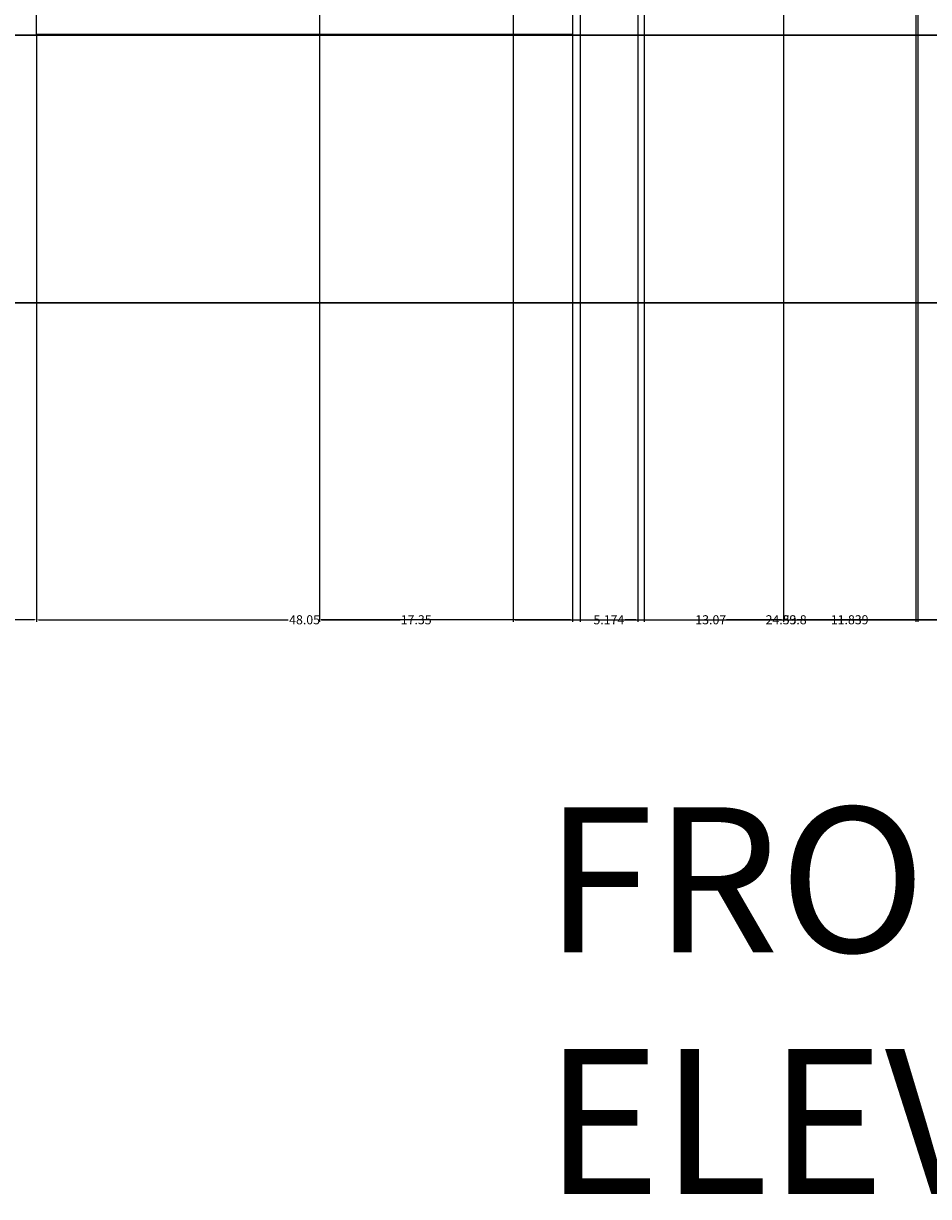
# Model space of a CAD drawing. Units: inches. Extents: x 69 to 650, y -16 to 573.
# Tile 4 of 26: x 264 to 345, y -16 to 89. Entities that reach past the tile are written whole.
import ezdxf

# ---------------------------------------------------------------- set-up
doc = ezdxf.new("R2010")
doc.units = ezdxf.units.IN
doc.header["$MEASUREMENT"] = 0
for name, color, linetype, lineweight in [('A-ANNO-DIMS', 2, 'Continuous', 18), ('A-ANNO-TEXT', 7, 'Continuous', 25), ('A-DOOR', 3, 'Continuous', 25), ('A-WALL-BASE', 7, 'Continuous', 30)]:
    doc.layers.add(name, color=color, linetype=linetype, lineweight=lineweight)
doc.styles.get("Standard").update_dxf_attribs({"font": 'arial.ttf'})
doc.dimstyles.get("Standard").update_dxf_attribs({"dimtxt": 0.8125, "dimasz": 0.18, "dimexe": 0.18, "dimexo": 0.0625, "dimgap": 0.09, "dimtad": 0, "dimtih": 1, "dimtoh": 1, "dimdec": 4, "dimzin": 0, "dimdsep": 46, "dimlunit": 4, "dimtxsty": 'Standard', "dimcen": 0.09, "dimadec": 0, "dimazin": 0, "dimtfac": 1, "dimtdec": 4, "dimtofl": 0, "dimtmove": 0, "dimatfit": 3, "dimfxl": 1, "dimtolj": 1, "dimtzin": 0, "dimarcsym": 0})

# ---------------------------------------------------------------- blocks, each defined once
blk = doc.blocks.new('*D19')
at = {"layer": 'A-ANNO-DIMS', "color": 0, "lineweight": -2, "transparency": 16777216}
for p, q in [((99.56, 471.72), (99.56, 572.74)), ((99.74, 572.56), (358.57, 572.56)), ((619.38, 572.56), (360.54, 572.56)), ((619.56, 87.99), (619.56, 572.74))]:
    blk.add_line(p, q, dxfattribs=at)
at = {"layer": 'A-ANNO-DIMS', "color": 0, "transparency": 16777216}
for points in [[(99.74, 572.59), (99.74, 572.53), (99.56, 572.56)], [(619.38, 572.59), (619.38, 572.53), (619.56, 572.56)]]:
    blk.add_solid(points, dxfattribs=at)
at = {"layer": 'Defpoints', "color": 0, "transparency": 16777216}
for p in [(619.56, 572.56), (99.56, 471.66), (619.56, 87.93)]:
    blk.add_point(p, dxfattribs=at)
at = {"layer": 'A-ANNO-DIMS', "color": 0, "transparency": 16777216, "insert": (359.56, 572.56), "char_height": 0.812, "attachment_point": 5}
blk.add_mtext('\\A1;520', dxfattribs=at)
blk = doc.blocks.new('*D28')
at = {"layer": 'A-ANNO-DIMS', "color": 0, "lineweight": -2, "transparency": 16777216}
for p, q in [((225, 87.87), (225, 35.35)), ((265.1, 87.92), (265.1, 35.35)), ((225.18, 35.53), (243.96, 35.53)), ((264.92, 35.53), (246.13, 35.53))]:
    blk.add_line(p, q, dxfattribs=at)
at = {"layer": 'A-ANNO-DIMS', "color": 0, "transparency": 16777216}
for points in [[(225.18, 35.56), (225.18, 35.5), (225, 35.53)], [(264.92, 35.56), (264.92, 35.5), (265.1, 35.53)]]:
    blk.add_solid(points, dxfattribs=at)
at = {"layer": 'Defpoints', "color": 0, "transparency": 16777216}
for p in [(225, 87.93), (265.1, 87.99), (265.1, 35.53)]:
    blk.add_point(p, dxfattribs=at)
at = {"layer": 'A-ANNO-DIMS', "color": 0, "transparency": 16777216, "insert": (245.05, 35.53), "char_height": 0.812, "attachment_point": 5}
blk.add_mtext('\\A1;40.1', dxfattribs=at)
blk = doc.blocks.new('*D29')
at = {"layer": 'A-ANNO-DIMS', "color": 0, "lineweight": -2, "transparency": 16777216}
for p, q in [((265.1, 87.92), (265.1, 35.35)), ((313.14, 87.92), (313.14, 35.35)), ((265.28, 35.53), (287.64, 35.53)), ((312.96, 35.53), (290.6, 35.53))]:
    blk.add_line(p, q, dxfattribs=at)
at = {"layer": 'A-ANNO-DIMS', "color": 0, "transparency": 16777216}
for points in [[(265.28, 35.56), (265.28, 35.5), (265.1, 35.53)], [(312.96, 35.56), (312.96, 35.5), (313.14, 35.53)]]:
    blk.add_solid(points, dxfattribs=at)
at = {"layer": 'Defpoints', "color": 0, "transparency": 16777216}
for p in [(265.1, 87.99), (313.14, 87.99), (313.14, 35.53)]:
    blk.add_point(p, dxfattribs=at)
at = {"layer": 'A-ANNO-DIMS', "color": 0, "transparency": 16777216, "insert": (289.12, 35.53), "char_height": 0.812, "attachment_point": 5}
blk.add_mtext('\\A1;48.05', dxfattribs=at)
blk = doc.blocks.new('*D30')
at = {"layer": 'A-ANNO-DIMS', "color": 0, "lineweight": -2, "transparency": 16777216}
for p, q in [((352.94, 174.2), (352.94, 35.35)), ((313.14, 87.92), (313.14, 35.35)), ((313.32, 35.53), (331.9, 35.53)), ((352.76, 35.53), (334.19, 35.53))]:
    blk.add_line(p, q, dxfattribs=at)
at = {"layer": 'A-ANNO-DIMS', "color": 0, "transparency": 16777216}
for points in [[(313.32, 35.56), (313.32, 35.5), (313.14, 35.53)], [(352.76, 35.56), (352.76, 35.5), (352.94, 35.53)]]:
    blk.add_solid(points, dxfattribs=at)
at = {"layer": 'Defpoints', "color": 0, "transparency": 16777216}
for p in [(352.94, 174.27), (313.14, 87.99), (352.94, 35.53)]:
    blk.add_point(p, dxfattribs=at)
at = {"layer": 'A-ANNO-DIMS', "color": 0, "transparency": 16777216, "insert": (333.04, 35.53), "char_height": 0.812, "attachment_point": 5}
blk.add_mtext('\\A1;39.8', dxfattribs=at)
blk = doc.blocks.new('*D37')
at = {"layer": 'A-ANNO-DIMS', "color": 0, "lineweight": -2, "transparency": 16777216}
for p, q in [((307.8, 384.84), (307.8, 35.35)), ((290.45, 372.93), (290.45, 35.35)), ((290.63, 35.53), (297.7, 35.53)), ((307.62, 35.53), (300.55, 35.53))]:
    blk.add_line(p, q, dxfattribs=at)
at = {"layer": 'A-ANNO-DIMS', "color": 0, "transparency": 16777216}
for points in [[(290.63, 35.56), (290.63, 35.5), (290.45, 35.53)], [(307.62, 35.56), (307.62, 35.5), (307.8, 35.53)]]:
    blk.add_solid(points, dxfattribs=at)
at = {"layer": 'Defpoints', "color": 0, "transparency": 16777216}
for p in [(307.8, 384.9), (290.45, 372.99), (307.8, 35.53)]:
    blk.add_point(p, dxfattribs=at)
at = {"layer": 'A-ANNO-DIMS', "color": 0, "transparency": 16777216, "insert": (299.12, 35.53), "char_height": 0.812, "attachment_point": 5}
blk.add_mtext('\\A1;17.35', dxfattribs=at)
blk = doc.blocks.new('*D38')
at = {"layer": 'A-ANNO-DIMS', "color": 0, "lineweight": -2, "transparency": 16777216}
for p, q in [((307.8, 384.84), (307.8, 35.35)), ((390.43, 384.84), (390.43, 35.35)), ((307.98, 35.53), (347.65, 35.53)), ((390.25, 35.53), (350.57, 35.53))]:
    blk.add_line(p, q, dxfattribs=at)
at = {"layer": 'A-ANNO-DIMS', "color": 0, "transparency": 16777216}
for points in [[(307.98, 35.56), (307.98, 35.5), (307.8, 35.53)], [(390.25, 35.56), (390.25, 35.5), (390.43, 35.53)]]:
    blk.add_solid(points, dxfattribs=at)
at = {"layer": 'Defpoints', "color": 0, "transparency": 16777216}
for p in [(307.8, 384.9), (390.43, 384.9), (390.43, 35.53)]:
    blk.add_point(p, dxfattribs=at)
at = {"layer": 'A-ANNO-DIMS', "color": 0, "transparency": 16777216, "insert": (349.11, 35.53), "char_height": 0.812, "attachment_point": 5}
blk.add_mtext('\\A1;82.63', dxfattribs=at)
blk = doc.blocks.new('*D64')
at = {"layer": 'A-ANNO-DIMS', "color": 0, "lineweight": -2, "transparency": 16777216}
for p, q in [((319.55, 393.8), (319.55, 35.35)), ((344.08, 393.8), (344.08, 35.35)), ((319.73, 35.53), (330.35, 35.53)), ((343.9, 35.53), (333.28, 35.53))]:
    blk.add_line(p, q, dxfattribs=at)
at = {"layer": 'A-ANNO-DIMS', "color": 0, "transparency": 16777216}
for points in [[(319.73, 35.56), (319.73, 35.5), (319.55, 35.53)], [(343.9, 35.56), (343.9, 35.5), (344.08, 35.53)]]:
    blk.add_solid(points, dxfattribs=at)
at = {"layer": 'Defpoints', "color": 0, "transparency": 16777216}
for p in [(319.55, 393.86), (344.08, 393.86), (344.08, 35.53)]:
    blk.add_point(p, dxfattribs=at)
at = {"layer": 'A-ANNO-DIMS', "color": 0, "transparency": 16777216, "insert": (331.82, 35.53), "char_height": 0.812, "attachment_point": 5}
blk.add_mtext('\\A1;24.53', dxfattribs=at)
blk = doc.blocks.new('*D65')
at = {"layer": 'A-ANNO-DIMS', "color": 0, "lineweight": -2, "transparency": 16777216}
for p, q in [((344.08, 393.8), (344.08, 35.35)), ((368.88, 393.8), (368.88, 35.35)), ((344.26, 35.53), (355.33, 35.53)), ((368.7, 35.53), (357.63, 35.53))]:
    blk.add_line(p, q, dxfattribs=at)
at = {"layer": 'A-ANNO-DIMS', "color": 0, "transparency": 16777216}
for points in [[(344.26, 35.56), (344.26, 35.5), (344.08, 35.53)], [(368.7, 35.56), (368.7, 35.5), (368.88, 35.53)]]:
    blk.add_solid(points, dxfattribs=at)
at = {"layer": 'Defpoints', "color": 0, "transparency": 16777216}
for p in [(344.08, 393.86), (368.88, 393.86), (368.88, 35.53)]:
    blk.add_point(p, dxfattribs=at)
at = {"layer": 'A-ANNO-DIMS', "color": 0, "transparency": 16777216, "insert": (356.48, 35.53), "char_height": 0.812, "attachment_point": 5}
blk.add_mtext('\\A1;24.8', dxfattribs=at)
blk = doc.blocks.new('*D66')
at = {"layer": 'A-ANNO-DIMS', "color": 0, "lineweight": -2, "transparency": 16777216}
for p, q in [((313.81, 263.46), (313.81, 35.35)), ((318.98, 263.46), (318.98, 35.35)), ((313.99, 35.53), (314.93, 35.53)), ((318.8, 35.53), (317.85, 35.53))]:
    blk.add_line(p, q, dxfattribs=at)
at = {"layer": 'A-ANNO-DIMS', "color": 0, "transparency": 16777216}
for points in [[(313.99, 35.56), (313.99, 35.5), (313.81, 35.53)], [(318.8, 35.56), (318.8, 35.5), (318.98, 35.53)]]:
    blk.add_solid(points, dxfattribs=at)
at = {"layer": 'Defpoints', "color": 0, "transparency": 16777216}
for p in [(313.81, 263.53), (318.98, 263.53), (318.98, 35.53)]:
    blk.add_point(p, dxfattribs=at)
at = {"layer": 'A-ANNO-DIMS', "color": 0, "transparency": 16777216, "insert": (316.39, 35.53), "char_height": 0.812, "attachment_point": 5}
blk.add_mtext('\\A1;5.174', dxfattribs=at)
blk = doc.blocks.new('*D67')
at = {"layer": 'A-ANNO-DIMS', "color": 0, "lineweight": -2, "transparency": 16777216}
for p, q in [((318.98, 263.46), (318.98, 35.35)), ((332.05, 263.46), (332.05, 35.35)), ((319.16, 35.53), (324.09, 35.53)), ((331.87, 35.53), (326.94, 35.53))]:
    blk.add_line(p, q, dxfattribs=at)
at = {"layer": 'A-ANNO-DIMS', "color": 0, "transparency": 16777216}
for points in [[(319.16, 35.56), (319.16, 35.5), (318.98, 35.53)], [(331.87, 35.56), (331.87, 35.5), (332.05, 35.53)]]:
    blk.add_solid(points, dxfattribs=at)
at = {"layer": 'Defpoints', "color": 0, "transparency": 16777216}
for p in [(318.98, 263.53), (332.05, 263.53), (332.05, 35.53)]:
    blk.add_point(p, dxfattribs=at)
at = {"layer": 'A-ANNO-DIMS', "color": 0, "transparency": 16777216, "insert": (325.52, 35.53), "char_height": 0.812, "attachment_point": 5}
blk.add_mtext('\\A1;13.07', dxfattribs=at)
blk = doc.blocks.new('*D68')
at = {"layer": 'A-ANNO-DIMS', "color": 0, "lineweight": -2, "transparency": 16777216}
for p, q in [((332.05, 263.46), (332.05, 35.35)), ((343.89, 263.46), (343.89, 35.35)), ((332.23, 35.53), (336.23, 35.53)), ((343.71, 35.53), (339.71, 35.53))]:
    blk.add_line(p, q, dxfattribs=at)
at = {"layer": 'A-ANNO-DIMS', "color": 0, "transparency": 16777216}
for points in [[(332.23, 35.56), (332.23, 35.5), (332.05, 35.53)], [(343.71, 35.56), (343.71, 35.5), (343.89, 35.53)]]:
    blk.add_solid(points, dxfattribs=at)
at = {"layer": 'Defpoints', "color": 0, "transparency": 16777216}
for p in [(332.05, 263.53), (343.89, 263.53), (343.89, 35.53)]:
    blk.add_point(p, dxfattribs=at)
at = {"layer": 'A-ANNO-DIMS', "color": 0, "transparency": 16777216, "insert": (337.97, 35.53), "char_height": 0.812, "attachment_point": 5}
blk.add_mtext('\\A1;11.839', dxfattribs=at)
blk = doc.blocks.new('*D69')
at = {"layer": 'A-ANNO-DIMS', "color": 0, "lineweight": -2, "transparency": 16777216}
for p, q in [((343.89, 263.46), (343.89, 35.35)), ((357.51, 263.46), (357.51, 35.35)), ((344.07, 35.53), (349.28, 35.53)), ((357.33, 35.53), (352.12, 35.53))]:
    blk.add_line(p, q, dxfattribs=at)
at = {"layer": 'A-ANNO-DIMS', "color": 0, "transparency": 16777216}
for points in [[(344.07, 35.56), (344.07, 35.5), (343.89, 35.53)], [(357.33, 35.56), (357.33, 35.5), (357.51, 35.53)]]:
    blk.add_solid(points, dxfattribs=at)
at = {"layer": 'Defpoints', "color": 0, "transparency": 16777216}
for p in [(343.89, 263.53), (357.51, 263.53), (357.51, 35.53)]:
    blk.add_point(p, dxfattribs=at)
at = {"layer": 'A-ANNO-DIMS', "color": 0, "transparency": 16777216, "insert": (350.7, 35.53), "char_height": 0.812, "attachment_point": 5}
blk.add_mtext('\\A1;13.62', dxfattribs=at)

msp = doc.modelspace()

# ---------------------------------------------------------------- linework, layer by layer
at = {"layer": 'A-DOOR'}
msp.add_lwpolyline([(265.0952, 174.2666), (313.1416, 174.2666), (313.1416, 87.985), (265.0952, 87.985)], close=True, dxfattribs=at)
at = {"layer": 'A-WALL-BASE'}
for p, q in [((99.556, 87.93), (463.7847, 87.93)), ((99.556, 63.93), (463.7847, 63.93))]:
    msp.add_line(p, q, dxfattribs=at)

# ---------------------------------------------------------------- texts
at = {"layer": 'A-ANNO-TEXT', "insert": (310.6022, 18.729), "char_height": 13, "attachment_point": 1}
msp.add_mtext_dynamic_manual_height_columns('FRONT ELEVATION', width=154.108417, gutter_width=1, heights=[0], dxfattribs=at)

# ---------------------------------------------------------------- dimensions: what is measured, and where the dimension line sits
at = {"layer": 'A-ANNO-DIMS'}
for base, p1, p2, override, picture, middle in [((619.555, 572.5573), (99.556, 471.6595), (619.555, 87.93), {"dimdec": 0, "dimlfac": 1, "dimrnd": 0, "dimzin": 0, "dimdsep": 46, "dimlunit": 2}, '*D19', (359.5555, 572.5573)), ((344.0804, 35.53), (319.5513, 393.8576), (344.0804, 393.8576), {"dimdec": 2, "dimlfac": 1, "dimrnd": 0, "dimzin": 0, "dimdsep": 46, "dimlunit": 2}, '*D64', (331.8159, 35.53)), ((368.881, 35.53), (344.0804, 393.8576), (368.881, 393.8576), {"dimdec": 1, "dimlfac": 1, "dimrnd": 0, "dimzin": 0, "dimdsep": 46, "dimlunit": 2}, '*D65', (356.4807, 35.53)), ((307.7955, 35.53), (290.4461, 372.9907), (307.7955, 384.8986), {"dimdec": 2, "dimlfac": 1, "dimrnd": 0, "dimzin": 0, "dimdsep": 46, "dimlunit": 2}, '*D37', (299.1208, 35.53)), ((390.4291, 35.53), (307.7955, 384.8986), (390.4291, 384.8986), {"dimdec": 2, "dimlfac": 1, "dimrnd": 0, "dimzin": 0, "dimdsep": 46, "dimlunit": 2}, '*D38', (349.1123, 35.53)), ((318.9804, 35.53), (313.8067, 263.5253), (318.9804, 263.5253), {"dimdec": 3, "dimlfac": 1, "dimrnd": 0, "dimzin": 0, "dimdsep": 46, "dimlunit": 2}, '*D66', (316.3936, 35.53)), ((332.0516, 35.53), (318.9804, 263.5253), (332.0516, 263.5253), {"dimdec": 2, "dimlfac": 1, "dimrnd": 0, "dimzin": 0, "dimdsep": 46, "dimlunit": 2}, '*D67', (325.516, 35.53)), ((343.8902, 35.53), (332.0516, 263.5253), (343.8902, 263.5253), {"dimdec": 3, "dimlfac": 1, "dimrnd": 0, "dimzin": 0, "dimdsep": 46, "dimlunit": 2}, '*D68', (337.9709, 35.53)), ((357.5106, 35.53), (343.8902, 263.5253), (357.5106, 263.5253), {"dimdec": 2, "dimlfac": 1, "dimrnd": 0, "dimzin": 0, "dimdsep": 46, "dimlunit": 2}, '*D69', (350.7004, 35.53)), ((352.9415, 35.53), (313.1416, 87.985), (352.9415, 174.2666), {"dimdec": 1, "dimlfac": 1, "dimrnd": 0, "dimzin": 0, "dimdsep": 46, "dimlunit": 2}, '*D30', (333.0415, 35.53)), ((265.0952, 35.53), (224.9972, 87.93), (265.0952, 87.985), {"dimdec": 1, "dimlfac": 1, "dimrnd": 0, "dimzin": 0, "dimdsep": 46, "dimlunit": 2}, '*D28', (245.0462, 35.53)), ((313.1416, 35.53), (265.0952, 87.985), (313.1416, 87.985), {"dimdec": 2, "dimlfac": 1, "dimrnd": 0, "dimzin": 0, "dimdsep": 46, "dimlunit": 2}, '*D29', (289.1184, 35.53))]:
    dim = msp.add_linear_dim(base=base, p1=p1, p2=p2, dimstyle='Standard', override=override, dxfattribs=at)
    dim.commit()
    dim.dimension.update_dxf_attribs({"geometry": picture, "text_midpoint": middle})

doc.saveas('drawing.dxf')
